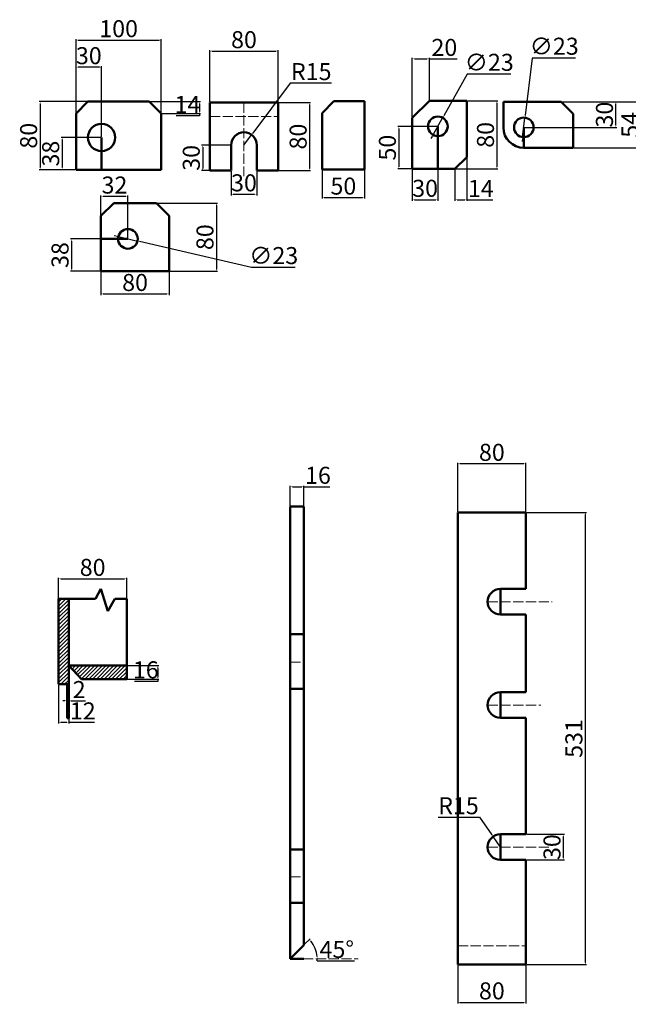
# Model space of a CAD drawing. Units: millimetres. Extents: x 1372 to 2780, y 1459 to 2779.
# Tile 1 of 2: x 1372 to 2087, y 1520 to 2676. Entities that reach past the tile are written whole.
import ezdxf

# ---------------------------------------------------------------- set-up
doc = ezdxf.new("R2010")
doc.units = ezdxf.units.MM
doc.linetypes.add('ACAD_ISO02W100', pattern=[15, 12, -3])
for name, color, linetype, lineweight in [('M-CNTR', 1, 'ACAD_ISO02W100', 18), ('M-DIMS', 2, 'Continuous', 25), ('M-HATC', 8, 'Continuous', 18), ('M-OUTL', 7, 'Continuous', 50)]:
    doc.layers.add(name, color=color, linetype=linetype, lineweight=lineweight)
doc.styles.get("Standard").update_dxf_attribs({"font": 'arial.ttf'})
doc.dimstyles.new('ISO-25', dxfattribs={"dimtxt": 20, "dimasz": 2.5, "dimexe": 1.25, "dimexo": 0.625, "dimtad": 1, "dimtoh": 1, "dimdec": 0, "dimtxsty": 'Standard', "dimcen": 2.5, "dimadec": 0, "dimazin": 0, "dimtfac": 1, "dimtdec": 0, "dimtmove": 0, "dimatfit": 3, "dimfxl": 1, "dimarcsym": 0})

# ---------------------------------------------------------------- blocks, each defined once
blk = doc.blocks.new('*D1')
at = {"layer": 'Defpoints', "color": 0, "transparency": 16777216}
for p in [(1705.8, 2128.1), (1689.8, 2105), (1705.8, 2105)]:
    blk.add_point(p, dxfattribs=at)
at = {"layer": 'M-DIMS', "color": 0, "lineweight": -2, "transparency": 16777216}
for p, q in [((1689.8, 2105.7), (1689.8, 2129.3)), ((1692.3, 2128.1), (1703.3, 2128.1)), ((1705.8, 2105.7), (1705.8, 2129.3)), ((1705.8, 2128.1), (1736.3, 2128.1))]:
    blk.add_line(p, q, dxfattribs=at)
at = {"layer": 'M-DIMS', "color": 0, "transparency": 16777216}
for points in [[(1692.3, 2128.5), (1692.3, 2127.7), (1689.8, 2128.1)], [(1703.3, 2128.5), (1703.3, 2127.7), (1705.8, 2128.1)]]:
    blk.add_solid(points, dxfattribs=at)
at = {"layer": 'M-DIMS', "color": 0, "transparency": 16777216, "insert": (1722.3, 2138.9), "char_height": 20, "attachment_point": 5}
blk.add_mtext('16', dxfattribs=at)
blk = doc.blocks.new('*D2')
at = {"layer": 'Defpoints', "color": 0, "transparency": 16777216}
for p in [(1705.8, 1590), (1717.1, 1589.8), (1689.8, 1574), (1689.8, 1574), (1769.4, 1574)]:
    blk.add_point(p, dxfattribs=at)
at = {"layer": 'M-DIMS', "color": 0, "lineweight": -2, "transparency": 16777216}
for p, q in [((1706.2, 1590.5), (1713, 1597.2)), ((1721.3, 1571.6), (1765.1, 1571.6))]:
    blk.add_line(p, q, dxfattribs=at)
for start, end in [(4.5402, 40.4598), (355.4598, 360)]:
    blk.add_arc((1689.8, 1574), 31.6, start, end, dxfattribs=at)
at = {"layer": 'M-DIMS', "color": 0, "transparency": 16777216}
for points in [[(1713.5, 1594.2), (1714.1, 1594.8), (1712.1, 1596.4)], [(1721.7, 1576.6), (1720.8, 1576.5), (1721.4, 1574)]]:
    blk.add_solid(points, dxfattribs=at)
at = {"layer": 'M-DIMS', "color": 0, "transparency": 16777216, "insert": (1744.4, 1582.3), "char_height": 20, "attachment_point": 5}
blk.add_mtext('45°', dxfattribs=at)
blk = doc.blocks.new('*D3')
at = {"layer": 'Defpoints', "color": 0, "transparency": 16777216}
for p in [(1497.7, 2019.9), (1417.7, 1996.3), (1497.7, 1996.3)]:
    blk.add_point(p, dxfattribs=at)
at = {"layer": 'M-DIMS', "color": 0, "lineweight": -2, "transparency": 16777216}
for p, q in [((1417.7, 1996.9), (1417.7, 2021.2)), ((1420.2, 2019.9), (1495.2, 2019.9)), ((1497.7, 1996.9), (1497.7, 2021.2))]:
    blk.add_line(p, q, dxfattribs=at)
at = {"layer": 'M-DIMS', "color": 0, "transparency": 16777216}
for points in [[(1420.2, 2020.3), (1420.2, 2019.5), (1417.7, 2019.9)], [(1495.2, 2020.3), (1495.2, 2019.5), (1497.7, 2019.9)]]:
    blk.add_solid(points, dxfattribs=at)
at = {"layer": 'M-DIMS', "color": 0, "transparency": 16777216, "insert": (1457.7, 2030.8), "char_height": 20, "attachment_point": 5}
blk.add_mtext('80', dxfattribs=at)
blk = doc.blocks.new('*D4')
at = {"layer": 'Defpoints', "color": 0, "transparency": 16777216}
for p in [(1497.7, 1918.1), (1497.7, 1902.1), (1534.1, 1902.1)]:
    blk.add_point(p, dxfattribs=at)
at = {"layer": 'M-DIMS', "color": 0, "lineweight": -2, "transparency": 16777216}
for p, q in [((1498.3, 1918.1), (1535.3, 1918.1)), ((1534.1, 1915.6), (1534.1, 1904.6)), ((1498.3, 1902.1), (1535.3, 1902.1)), ((1534.1, 1899.6), (1506.7, 1899.6)), ((1534.1, 1902.1), (1534.1, 1899.6))]:
    blk.add_line(p, q, dxfattribs=at)
at = {"layer": 'M-DIMS', "color": 0, "transparency": 16777216}
for points in [[(1533.7, 1915.6), (1534.5, 1915.6), (1534.1, 1918.1)], [(1533.7, 1904.6), (1534.5, 1904.6), (1534.1, 1902.1)]]:
    blk.add_solid(points, dxfattribs=at)
at = {"layer": 'M-DIMS', "color": 0, "transparency": 16777216, "insert": (1520.1, 1910.5), "char_height": 20, "attachment_point": 5}
blk.add_mtext('16', dxfattribs=at)
blk = doc.blocks.new('*D5')
at = {"layer": 'Defpoints', "color": 0, "transparency": 16777216}
for p in [(1417.7, 1896.3), (1429.7, 1896.3), (1429.7, 1851.6)]:
    blk.add_point(p, dxfattribs=at)
at = {"layer": 'M-DIMS', "color": 0, "lineweight": -2, "transparency": 16777216}
for p, q in [((1417.7, 1895.7), (1417.7, 1850.3)), ((1429.7, 1895.7), (1429.7, 1850.3)), ((1420.2, 1851.6), (1427.2, 1851.6)), ((1429.7, 1851.6), (1460, 1851.6))]:
    blk.add_line(p, q, dxfattribs=at)
at = {"layer": 'M-DIMS', "color": 0, "transparency": 16777216}
for points in [[(1420.2, 1852), (1420.2, 1851.2), (1417.7, 1851.6)], [(1427.2, 1852), (1427.2, 1851.2), (1429.7, 1851.6)]]:
    blk.add_solid(points, dxfattribs=at)
at = {"layer": 'M-DIMS', "color": 0, "transparency": 16777216, "insert": (1446.1, 1862.3), "char_height": 20, "attachment_point": 5}
blk.add_mtext('12', dxfattribs=at)
blk = doc.blocks.new('*D6')
at = {"layer": 'Defpoints', "color": 0, "transparency": 16777216}
for p in [(1429.7, 1876.8), (1427.7, 1856.3), (1429.7, 1856.3)]:
    blk.add_point(p, dxfattribs=at)
at = {"layer": 'M-DIMS', "color": 0, "lineweight": -2, "transparency": 16777216}
for p, q in [((1425.2, 1876.8), (1422.7, 1876.8)), ((1427.7, 1856.9), (1427.7, 1878)), ((1427.7, 1876.8), (1429.7, 1876.8)), ((1429.7, 1856.9), (1429.7, 1878)), ((1432.2, 1876.8), (1449.2, 1876.8))]:
    blk.add_line(p, q, dxfattribs=at)
at = {"layer": 'M-DIMS', "color": 0, "transparency": 16777216}
for points in [[(1425.2, 1877.2), (1425.2, 1876.3), (1427.7, 1876.8)], [(1432.2, 1877.2), (1432.2, 1876.3), (1429.7, 1876.8)]]:
    blk.add_solid(points, dxfattribs=at)
at = {"layer": 'M-DIMS', "color": 0, "transparency": 16777216, "insert": (1441.9, 1887.4), "char_height": 20, "attachment_point": 5}
blk.add_mtext('2', dxfattribs=at)
blk = doc.blocks.new('*D7')
at = {"layer": 'Defpoints', "color": 0, "transparency": 16777216}
for p in [(1886.5, 1567), (1966.5, 1567), (1966.5, 1522.7)]:
    blk.add_point(p, dxfattribs=at)
at = {"layer": 'M-DIMS', "color": 0, "lineweight": -2, "transparency": 16777216}
for p, q in [((1886.5, 1566.4), (1886.5, 1521.5)), ((1966.5, 1566.4), (1966.5, 1521.5)), ((1889, 1522.7), (1964, 1522.7))]:
    blk.add_line(p, q, dxfattribs=at)
at = {"layer": 'M-DIMS', "color": 0, "transparency": 16777216}
for points in [[(1889, 1523.1), (1889, 1522.3), (1886.5, 1522.7)], [(1964, 1523.1), (1964, 1522.3), (1966.5, 1522.7)]]:
    blk.add_solid(points, dxfattribs=at)
at = {"layer": 'M-DIMS', "color": 0, "transparency": 16777216, "insert": (1926.5, 1533.6), "char_height": 20, "attachment_point": 5}
blk.add_mtext('80', dxfattribs=at)
blk = doc.blocks.new('*D8')
at = {"layer": 'Defpoints', "color": 0, "transparency": 16777216}
for p in [(1966.5, 2098), (1966.5, 1567), (2036.2, 1567)]:
    blk.add_point(p, dxfattribs=at)
at = {"layer": 'M-DIMS', "color": 0, "lineweight": -2, "transparency": 16777216}
for p, q in [((1967.1, 2098), (2037.5, 2098)), ((2036.2, 2095.5), (2036.2, 1569.5)), ((1967.1, 1567), (2037.5, 1567))]:
    blk.add_line(p, q, dxfattribs=at)
at = {"layer": 'M-DIMS', "color": 0, "transparency": 16777216}
for points in [[(2035.8, 2095.5), (2036.7, 2095.5), (2036.2, 2098)], [(2035.8, 1569.5), (2036.7, 1569.5), (2036.2, 1567)]]:
    blk.add_solid(points, dxfattribs=at)
at = {"layer": 'M-DIMS', "color": 0, "transparency": 16777216, "insert": (2025.4, 1832.5), "char_height": 20, "attachment_point": 5, "rotation": 90}
blk.add_mtext('531', dxfattribs=at)
blk = doc.blocks.new('*D9')
at = {"layer": 'Defpoints', "color": 0, "transparency": 16777216}
for p in [(1966.5, 1720), (2010.6, 1720), (1966.5, 1690)]:
    blk.add_point(p, dxfattribs=at)
at = {"layer": 'M-DIMS', "color": 0, "lineweight": -2, "transparency": 16777216}
for p, q in [((1967.1, 1720), (2011.8, 1720)), ((2010.6, 1692.5), (2010.6, 1717.5)), ((1967.1, 1690), (2011.8, 1690))]:
    blk.add_line(p, q, dxfattribs=at)
at = {"layer": 'M-DIMS', "color": 0, "transparency": 16777216}
for points in [[(2010.1, 1717.5), (2011, 1717.5), (2010.6, 1720)], [(2010.1, 1692.5), (2011, 1692.5), (2010.6, 1690)]]:
    blk.add_solid(points, dxfattribs=at)
at = {"layer": 'M-DIMS', "color": 0, "transparency": 16777216, "insert": (1999.7, 1705), "char_height": 20, "attachment_point": 5, "rotation": 90}
blk.add_mtext('30', dxfattribs=at)
blk = doc.blocks.new('*D10')
at = {"layer": 'Defpoints', "color": 0, "transparency": 16777216}
for p in [(1927.9, 1717.3), (1936.5, 1705)]:
    blk.add_point(p, dxfattribs=at)
at = {"layer": 'M-DIMS', "color": 0, "lineweight": -2, "transparency": 16777216}
for p, q in [((1863.3, 1740.1), (1911.9, 1740.1)), ((1911.9, 1740.1), (1926.5, 1719.3)), ((1936.5, 1705), (1927.9, 1717.3))]:
    blk.add_line(p, q, dxfattribs=at)
at = {"layer": 'M-DIMS', "color": 0, "transparency": 16777216}
blk.add_solid([(1926.8, 1719.6), (1926.1, 1719.1), (1927.9, 1717.3)], dxfattribs=at)
at = {"layer": 'M-DIMS', "color": 0, "transparency": 16777216, "insert": (1887.3, 1751), "char_height": 20, "attachment_point": 5}
blk.add_mtext('R15', dxfattribs=at)
blk = doc.blocks.new('*D11')
at = {"layer": 'Defpoints', "color": 0, "transparency": 16777216}
for p in [(1886.5, 2155), (1886.5, 2098), (1966.5, 2098)]:
    blk.add_point(p, dxfattribs=at)
at = {"layer": 'M-DIMS', "color": 0, "lineweight": -2, "transparency": 16777216}
for p, q in [((1886.5, 2098.6), (1886.5, 2156.3)), ((1964, 2155), (1889, 2155)), ((1966.5, 2098.6), (1966.5, 2156.3))]:
    blk.add_line(p, q, dxfattribs=at)
at = {"layer": 'M-DIMS', "color": 0, "transparency": 16777216}
for points in [[(1889, 2155.4), (1889, 2154.6), (1886.5, 2155)], [(1964, 2155.4), (1964, 2154.6), (1966.5, 2155)]]:
    blk.add_solid(points, dxfattribs=at)
at = {"layer": 'M-DIMS', "color": 0, "transparency": 16777216, "insert": (1926.5, 2165.9), "char_height": 20, "attachment_point": 5}
blk.add_mtext('80', dxfattribs=at)
blk = doc.blocks.new('*D27')
at = {"layer": 'Defpoints', "color": 0, "transparency": 16777216}
for p in [(1467.5, 2381.1), (1547.5, 2381.1), (1547.5, 2354.5)]:
    blk.add_point(p, dxfattribs=at)
at = {"layer": 'M-DIMS', "color": 0, "lineweight": -2, "transparency": 16777216}
for p, q in [((1467.5, 2380.5), (1467.5, 2353.2)), ((1547.5, 2380.5), (1547.5, 2353.2)), ((1470, 2354.5), (1545, 2354.5))]:
    blk.add_line(p, q, dxfattribs=at)
at = {"layer": 'M-DIMS', "color": 0, "transparency": 16777216}
for points in [[(1470, 2354.9), (1470, 2354.1), (1467.5, 2354.5)], [(1545, 2354.9), (1545, 2354.1), (1547.5, 2354.5)]]:
    blk.add_solid(points, dxfattribs=at)
at = {"layer": 'M-DIMS', "color": 0, "transparency": 16777216, "insert": (1507.5, 2365.3), "char_height": 20, "attachment_point": 5}
blk.add_mtext('80', dxfattribs=at)
blk = doc.blocks.new('*D28')
at = {"layer": 'Defpoints', "color": 0, "transparency": 16777216}
for p in [(1499.1, 2419.1), (1432.9, 2381.1), (1467.5, 2381.1)]:
    blk.add_point(p, dxfattribs=at)
at = {"layer": 'M-DIMS', "color": 0, "lineweight": -2, "transparency": 16777216}
for p, q in [((1498.5, 2419.1), (1431.6, 2419.1)), ((1432.9, 2416.6), (1432.9, 2383.6)), ((1466.9, 2381.1), (1431.6, 2381.1))]:
    blk.add_line(p, q, dxfattribs=at)
at = {"layer": 'M-DIMS', "color": 0, "transparency": 16777216}
for points in [[(1432.4, 2416.6), (1433.3, 2416.6), (1432.9, 2419.1)], [(1432.4, 2383.6), (1433.3, 2383.6), (1432.9, 2381.1)]]:
    blk.add_solid(points, dxfattribs=at)
at = {"layer": 'M-DIMS', "color": 0, "transparency": 16777216, "insert": (1422, 2400.1), "char_height": 20, "attachment_point": 5, "rotation": 90}
blk.add_mtext('38', dxfattribs=at)
blk = doc.blocks.new('*D29')
at = {"layer": 'Defpoints', "color": 0, "transparency": 16777216}
for p in [(1467.5, 2468.9), (1467.5, 2446.1), (1499.1, 2419.1)]:
    blk.add_point(p, dxfattribs=at)
at = {"layer": 'M-DIMS', "color": 0, "lineweight": -2, "transparency": 16777216}
for p, q in [((1467.5, 2446.7), (1467.5, 2470.1)), ((1496.6, 2468.9), (1470, 2468.9)), ((1499.1, 2419.7), (1499.1, 2470.1))]:
    blk.add_line(p, q, dxfattribs=at)
at = {"layer": 'M-DIMS', "color": 0, "transparency": 16777216}
for points in [[(1470, 2469.3), (1470, 2468.5), (1467.5, 2468.9)], [(1496.6, 2469.3), (1496.6, 2468.5), (1499.1, 2468.9)]]:
    blk.add_solid(points, dxfattribs=at)
at = {"layer": 'M-DIMS', "color": 0, "transparency": 16777216, "insert": (1483.3, 2479.7), "char_height": 20, "attachment_point": 5}
blk.add_mtext('32', dxfattribs=at)
blk = doc.blocks.new('*D30')
at = {"layer": 'Defpoints', "color": 0, "transparency": 16777216}
for p in [(1532.5, 2461.1), (1547.5, 2381.1), (1603, 2381.1)]:
    blk.add_point(p, dxfattribs=at)
at = {"layer": 'M-DIMS', "color": 0, "lineweight": -2, "transparency": 16777216}
for p, q in [((1533.1, 2461.1), (1604.3, 2461.1)), ((1603, 2458.6), (1603, 2383.6)), ((1548.1, 2381.1), (1604.3, 2381.1))]:
    blk.add_line(p, q, dxfattribs=at)
at = {"layer": 'M-DIMS', "color": 0, "transparency": 16777216}
for points in [[(1602.6, 2458.6), (1603.4, 2458.6), (1603, 2461.1)], [(1602.6, 2383.6), (1603.4, 2383.6), (1603, 2381.1)]]:
    blk.add_solid(points, dxfattribs=at)
at = {"layer": 'M-DIMS', "color": 0, "transparency": 16777216, "insert": (1592.2, 2421.1), "char_height": 20, "attachment_point": 5, "rotation": 90}
blk.add_mtext('80', dxfattribs=at)
blk = doc.blocks.new('*D31')
at = {"layer": 'Defpoints', "color": 0, "transparency": 16777216}
for p in [(1487.9, 2421.7), (1510.3, 2416.5)]:
    blk.add_point(p, dxfattribs=at)
at = {"layer": 'M-DIMS', "color": 0, "lineweight": -2, "transparency": 16777216}
for p, q in [((1485.5, 2422.2), (1483.1, 2422.8)), ((1487.9, 2421.7), (1510.3, 2416.5)), ((1644.4, 2385.5), (1512.8, 2415.9)), ((1695.5, 2385.5), (1644.4, 2385.5))]:
    blk.add_line(p, q, dxfattribs=at)
at = {"layer": 'M-DIMS', "color": 0, "transparency": 16777216}
for points in [[(1485.6, 2422.6), (1485.4, 2421.8), (1487.9, 2421.7)], [(1512.9, 2416.3), (1512.7, 2415.5), (1510.3, 2416.5)]]:
    blk.add_solid(points, dxfattribs=at)
at = {"layer": 'M-DIMS', "color": 0, "transparency": 16777216, "insert": (1670.3, 2396.9), "char_height": 20, "attachment_point": 5}
blk.add_mtext('∅23', dxfattribs=at)
blk = doc.blocks.new('*D32')
at = {"layer": 'Defpoints', "color": 0, "transparency": 16777216}
for p in [(1438.2, 2620.8), (1438.2, 2533.2), (1468.2, 2538.2)]:
    blk.add_point(p, dxfattribs=at)
at = {"layer": 'M-DIMS', "color": 0, "lineweight": -2, "transparency": 16777216}
for p, q in [((1438.2, 2533.8), (1438.2, 2622)), ((1465.7, 2620.8), (1440.7, 2620.8)), ((1468.2, 2538.8), (1468.2, 2622))]:
    blk.add_line(p, q, dxfattribs=at)
at = {"layer": 'M-DIMS', "color": 0, "transparency": 16777216}
for points in [[(1440.7, 2621.2), (1440.7, 2620.4), (1438.2, 2620.8)], [(1465.7, 2621.2), (1465.7, 2620.4), (1468.2, 2620.8)]]:
    blk.add_solid(points, dxfattribs=at)
at = {"layer": 'M-DIMS', "color": 0, "transparency": 16777216, "insert": (1453.2, 2631.6), "char_height": 20, "attachment_point": 5}
blk.add_mtext('30', dxfattribs=at)
blk = doc.blocks.new('*D33')
at = {"layer": 'Defpoints', "color": 0, "transparency": 16777216}
for p in [(1524.2, 2580.2), (1538.2, 2566.2), (1583, 2566.2)]:
    blk.add_point(p, dxfattribs=at)
at = {"layer": 'M-DIMS', "color": 0, "lineweight": -2, "transparency": 16777216}
for p, q in [((1524.8, 2580.2), (1584.2, 2580.2)), ((1583, 2577.7), (1583, 2568.7)), ((1538.8, 2566.2), (1584.2, 2566.2)), ((1583, 2563.7), (1555.6, 2563.7)), ((1583, 2566.2), (1583, 2563.7))]:
    blk.add_line(p, q, dxfattribs=at)
at = {"layer": 'M-DIMS', "color": 0, "transparency": 16777216}
for points in [[(1582.5, 2577.7), (1583.4, 2577.7), (1583, 2580.2)], [(1582.5, 2568.7), (1583.4, 2568.7), (1583, 2566.2)]]:
    blk.add_solid(points, dxfattribs=at)
at = {"layer": 'M-DIMS', "color": 0, "transparency": 16777216, "insert": (1569, 2574.3), "char_height": 20, "attachment_point": 5}
blk.add_mtext('14', dxfattribs=at)
blk = doc.blocks.new('*D34')
at = {"layer": 'Defpoints', "color": 0, "transparency": 16777216}
for p in [(1452.2, 2580.2), (1396, 2500.2), (1438.2, 2500.2)]:
    blk.add_point(p, dxfattribs=at)
at = {"layer": 'M-DIMS', "color": 0, "lineweight": -2, "transparency": 16777216}
for p, q in [((1451.6, 2580.2), (1394.7, 2580.2)), ((1396, 2577.7), (1396, 2502.7)), ((1437.6, 2500.2), (1394.7, 2500.2))]:
    blk.add_line(p, q, dxfattribs=at)
at = {"layer": 'M-DIMS', "color": 0, "transparency": 16777216}
for points in [[(1395.6, 2577.7), (1396.4, 2577.7), (1396, 2580.2)], [(1395.6, 2502.7), (1396.4, 2502.7), (1396, 2500.2)]]:
    blk.add_solid(points, dxfattribs=at)
at = {"layer": 'M-DIMS', "color": 0, "transparency": 16777216, "insert": (1385.1, 2540.2), "char_height": 20, "attachment_point": 5, "rotation": 90}
blk.add_mtext('80', dxfattribs=at)
blk = doc.blocks.new('*D35')
at = {"layer": 'Defpoints', "color": 0, "transparency": 16777216}
for p in [(1468.2, 2538.2), (1421.9, 2500.2), (1438.2, 2500.2)]:
    blk.add_point(p, dxfattribs=at)
at = {"layer": 'M-DIMS', "color": 0, "lineweight": -2, "transparency": 16777216}
for p, q in [((1467.6, 2538.2), (1420.6, 2538.2)), ((1421.9, 2535.7), (1421.9, 2502.7)), ((1437.6, 2500.2), (1420.6, 2500.2))]:
    blk.add_line(p, q, dxfattribs=at)
at = {"layer": 'M-DIMS', "color": 0, "transparency": 16777216}
for points in [[(1421.4, 2535.7), (1422.3, 2535.7), (1421.9, 2538.2)], [(1421.4, 2502.7), (1422.3, 2502.7), (1421.9, 2500.2)]]:
    blk.add_solid(points, dxfattribs=at)
at = {"layer": 'M-DIMS', "color": 0, "transparency": 16777216, "insert": (1411, 2519.2), "char_height": 20, "attachment_point": 5, "rotation": 90}
blk.add_mtext('38', dxfattribs=at)
blk = doc.blocks.new('*D36')
at = {"layer": 'Defpoints', "color": 0, "transparency": 16777216}
for p in [(1538.2, 2652.5), (1438.2, 2500.2), (1538.2, 2500.2)]:
    blk.add_point(p, dxfattribs=at)
at = {"layer": 'M-DIMS', "color": 0, "lineweight": -2, "transparency": 16777216}
for p, q in [((1438.2, 2500.8), (1438.2, 2653.7)), ((1440.7, 2652.5), (1535.7, 2652.5)), ((1538.2, 2500.8), (1538.2, 2653.7))]:
    blk.add_line(p, q, dxfattribs=at)
at = {"layer": 'M-DIMS', "color": 0, "transparency": 16777216}
for points in [[(1440.7, 2652.9), (1440.7, 2652.1), (1438.2, 2652.5)], [(1535.7, 2652.9), (1535.7, 2652.1), (1538.2, 2652.5)]]:
    blk.add_solid(points, dxfattribs=at)
at = {"layer": 'M-DIMS', "color": 0, "transparency": 16777216, "insert": (1488.2, 2663.3), "char_height": 20, "attachment_point": 5}
blk.add_mtext('100', dxfattribs=at)
blk = doc.blocks.new('*D37')
at = {"layer": 'Defpoints', "color": 0, "transparency": 16777216}
for p in [(1675.4, 2639.6), (1595.4, 2579.2), (1675.4, 2579.2)]:
    blk.add_point(p, dxfattribs=at)
at = {"layer": 'M-DIMS', "color": 0, "lineweight": -2, "transparency": 16777216}
for p, q in [((1595.4, 2579.8), (1595.4, 2640.8)), ((1597.9, 2639.6), (1672.9, 2639.6)), ((1675.4, 2579.8), (1675.4, 2640.8))]:
    blk.add_line(p, q, dxfattribs=at)
at = {"layer": 'M-DIMS', "color": 0, "transparency": 16777216}
for points in [[(1597.9, 2640), (1597.9, 2639.1), (1595.4, 2639.6)], [(1672.9, 2640), (1672.9, 2639.1), (1675.4, 2639.6)]]:
    blk.add_solid(points, dxfattribs=at)
at = {"layer": 'M-DIMS', "color": 0, "transparency": 16777216, "insert": (1635.4, 2650.4), "char_height": 20, "attachment_point": 5}
blk.add_mtext('80', dxfattribs=at)
blk = doc.blocks.new('*D38')
at = {"layer": 'Defpoints', "color": 0, "transparency": 16777216}
for p in [(1675.4, 2579.2), (1675.4, 2499.2), (1712.4, 2499.2)]:
    blk.add_point(p, dxfattribs=at)
at = {"layer": 'M-DIMS', "color": 0, "lineweight": -2, "transparency": 16777216}
for p, q in [((1676, 2579.2), (1713.7, 2579.2)), ((1712.4, 2576.7), (1712.4, 2501.7)), ((1676, 2499.2), (1713.7, 2499.2))]:
    blk.add_line(p, q, dxfattribs=at)
at = {"layer": 'M-DIMS', "color": 0, "transparency": 16777216}
for points in [[(1712, 2576.7), (1712.8, 2576.7), (1712.4, 2579.2)], [(1712, 2501.7), (1712.8, 2501.7), (1712.4, 2499.2)]]:
    blk.add_solid(points, dxfattribs=at)
at = {"layer": 'M-DIMS', "color": 0, "transparency": 16777216, "insert": (1701.6, 2539.2), "char_height": 20, "attachment_point": 5, "rotation": 90}
blk.add_mtext('80', dxfattribs=at)
blk = doc.blocks.new('*D39')
at = {"layer": 'Defpoints', "color": 0, "transparency": 16777216}
for p in [(1620.4, 2499.2), (1650.4, 2499.2), (1650.4, 2471.5)]:
    blk.add_point(p, dxfattribs=at)
at = {"layer": 'M-DIMS', "color": 0, "lineweight": -2, "transparency": 16777216}
for p, q in [((1620.4, 2498.6), (1620.4, 2470.2)), ((1650.4, 2498.6), (1650.4, 2470.2)), ((1622.9, 2471.5), (1647.9, 2471.5))]:
    blk.add_line(p, q, dxfattribs=at)
at = {"layer": 'M-DIMS', "color": 0, "transparency": 16777216}
for points in [[(1622.9, 2471.9), (1622.9, 2471.1), (1620.4, 2471.5)], [(1647.9, 2471.9), (1647.9, 2471.1), (1650.4, 2471.5)]]:
    blk.add_solid(points, dxfattribs=at)
at = {"layer": 'M-DIMS', "color": 0, "transparency": 16777216, "insert": (1635.4, 2482.3), "char_height": 20, "attachment_point": 5}
blk.add_mtext('30', dxfattribs=at)
blk = doc.blocks.new('*D40')
at = {"layer": 'Defpoints', "color": 0, "transparency": 16777216}
for p in [(1644.3, 2541.2), (1635.4, 2529.2)]:
    blk.add_point(p, dxfattribs=at)
at = {"layer": 'M-DIMS', "color": 0, "lineweight": -2, "transparency": 16777216}
for p, q in [((1689.8, 2602.1), (1645.8, 2543.2)), ((1738.3, 2602.1), (1689.8, 2602.1)), ((1635.4, 2529.2), (1644.3, 2541.2))]:
    blk.add_line(p, q, dxfattribs=at)
at = {"layer": 'M-DIMS', "color": 0, "transparency": 16777216}
blk.add_solid([(1645.5, 2543.5), (1646.2, 2543), (1644.3, 2541.2)], dxfattribs=at)
at = {"layer": 'M-DIMS', "color": 0, "transparency": 16777216, "insert": (1714.4, 2612.9), "char_height": 20, "attachment_point": 5}
blk.add_mtext('R15', dxfattribs=at)
blk = doc.blocks.new('*D41')
at = {"layer": 'Defpoints', "color": 0, "transparency": 16777216}
for p in [(1620.4, 2529.2), (1586.9, 2499.2), (1620.4, 2499.2)]:
    blk.add_point(p, dxfattribs=at)
at = {"layer": 'M-DIMS', "color": 0, "lineweight": -2, "transparency": 16777216}
for p, q in [((1619.7, 2529.2), (1585.7, 2529.2)), ((1586.9, 2526.7), (1586.9, 2501.7)), ((1619.7, 2499.2), (1585.7, 2499.2))]:
    blk.add_line(p, q, dxfattribs=at)
at = {"layer": 'M-DIMS', "color": 0, "transparency": 16777216}
for points in [[(1586.5, 2526.7), (1587.3, 2526.7), (1586.9, 2529.2)], [(1586.5, 2501.7), (1587.3, 2501.7), (1586.9, 2499.2)]]:
    blk.add_solid(points, dxfattribs=at)
at = {"layer": 'M-DIMS', "color": 0, "transparency": 16777216, "insert": (1576.1, 2514.2), "char_height": 20, "attachment_point": 5, "rotation": 90}
blk.add_mtext('30', dxfattribs=at)
blk = doc.blocks.new('*D42')
at = {"layer": 'Defpoints', "color": 0, "transparency": 16777216}
for p in [(1727.1, 2500.6), (1777.1, 2500.6), (1777.1, 2467.6)]:
    blk.add_point(p, dxfattribs=at)
at = {"layer": 'M-DIMS', "color": 0, "lineweight": -2, "transparency": 16777216}
for p, q in [((1727.1, 2500), (1727.1, 2466.4)), ((1777.1, 2500), (1777.1, 2466.4)), ((1729.6, 2467.6), (1774.6, 2467.6))]:
    blk.add_line(p, q, dxfattribs=at)
at = {"layer": 'M-DIMS', "color": 0, "transparency": 16777216}
for points in [[(1729.6, 2468), (1729.6, 2467.2), (1727.1, 2467.6)], [(1774.6, 2468), (1774.6, 2467.2), (1777.1, 2467.6)]]:
    blk.add_solid(points, dxfattribs=at)
at = {"layer": 'M-DIMS', "color": 0, "transparency": 16777216, "insert": (1752.1, 2478.5), "char_height": 20, "attachment_point": 5}
blk.add_mtext('50', dxfattribs=at)
blk = doc.blocks.new('*D43')
at = {"layer": 'Defpoints', "color": 0, "transparency": 16777216}
for p in [(1833.1, 2501.2), (1863.1, 2501.2), (1863.1, 2465)]:
    blk.add_point(p, dxfattribs=at)
at = {"layer": 'M-DIMS', "color": 0, "lineweight": -2, "transparency": 16777216}
for p, q in [((1833.1, 2500.6), (1833.1, 2463.8)), ((1863.1, 2500.6), (1863.1, 2463.8)), ((1835.6, 2465), (1860.6, 2465))]:
    blk.add_line(p, q, dxfattribs=at)
at = {"layer": 'M-DIMS', "color": 0, "transparency": 16777216}
for points in [[(1835.6, 2465.4), (1835.6, 2464.6), (1833.1, 2465)], [(1860.6, 2465.4), (1860.6, 2464.6), (1863.1, 2465)]]:
    blk.add_solid(points, dxfattribs=at)
at = {"layer": 'M-DIMS', "color": 0, "transparency": 16777216, "insert": (1848.1, 2475.9), "char_height": 20, "attachment_point": 5}
blk.add_mtext('30', dxfattribs=at)
blk = doc.blocks.new('*D44')
at = {"layer": 'Defpoints', "color": 0, "transparency": 16777216}
for p in [(1853.1, 2630.5), (1853.1, 2581.2), (1833.1, 2561.2)]:
    blk.add_point(p, dxfattribs=at)
at = {"layer": 'M-DIMS', "color": 0, "lineweight": -2, "transparency": 16777216}
for p, q in [((1833.1, 2561.9), (1833.1, 2631.8)), ((1835.6, 2630.5), (1850.6, 2630.5)), ((1853.1, 2581.9), (1853.1, 2631.8)), ((1853.1, 2630.5), (1885.8, 2630.5))]:
    blk.add_line(p, q, dxfattribs=at)
at = {"layer": 'M-DIMS', "color": 0, "transparency": 16777216}
for points in [[(1835.6, 2630.9), (1835.6, 2630.1), (1833.1, 2630.5)], [(1850.6, 2630.9), (1850.6, 2630.1), (1853.1, 2630.5)]]:
    blk.add_solid(points, dxfattribs=at)
at = {"layer": 'M-DIMS', "color": 0, "transparency": 16777216, "insert": (1870.7, 2641.3), "char_height": 20, "attachment_point": 5}
blk.add_mtext('20', dxfattribs=at)
blk = doc.blocks.new('*D45')
at = {"layer": 'Defpoints', "color": 0, "transparency": 16777216}
for p in [(1897.1, 2515.2), (1883.1, 2501.2), (1897.1, 2465)]:
    blk.add_point(p, dxfattribs=at)
at = {"layer": 'M-DIMS', "color": 0, "lineweight": -2, "transparency": 16777216}
for p, q in [((1897.1, 2514.6), (1897.1, 2463.8)), ((1883.1, 2500.6), (1883.1, 2463.8)), ((1885.6, 2465), (1894.6, 2465)), ((1897.1, 2465), (1927.5, 2465))]:
    blk.add_line(p, q, dxfattribs=at)
at = {"layer": 'M-DIMS', "color": 0, "transparency": 16777216}
for points in [[(1885.6, 2465.4), (1885.6, 2464.6), (1883.1, 2465)], [(1894.6, 2465.4), (1894.6, 2464.6), (1897.1, 2465)]]:
    blk.add_solid(points, dxfattribs=at)
at = {"layer": 'M-DIMS', "color": 0, "transparency": 16777216, "insert": (1913.6, 2475.7), "char_height": 20, "attachment_point": 5}
blk.add_mtext('14', dxfattribs=at)
blk = doc.blocks.new('*D46')
at = {"layer": 'Defpoints', "color": 0, "transparency": 16777216}
for p in [(1897.1, 2581.2), (1883.1, 2501.2), (1932.4, 2501.2)]:
    blk.add_point(p, dxfattribs=at)
at = {"layer": 'M-DIMS', "color": 0, "lineweight": -2, "transparency": 16777216}
for p, q in [((1897.7, 2581.2), (1933.6, 2581.2)), ((1932.4, 2578.7), (1932.4, 2503.7)), ((1883.7, 2501.2), (1933.6, 2501.2))]:
    blk.add_line(p, q, dxfattribs=at)
at = {"layer": 'M-DIMS', "color": 0, "transparency": 16777216}
for points in [[(1932, 2578.7), (1932.8, 2578.7), (1932.4, 2581.2)], [(1932, 2503.7), (1932.8, 2503.7), (1932.4, 2501.2)]]:
    blk.add_solid(points, dxfattribs=at)
at = {"layer": 'M-DIMS', "color": 0, "transparency": 16777216, "insert": (1921.6, 2541.2), "char_height": 20, "attachment_point": 5, "rotation": 90}
blk.add_mtext('80', dxfattribs=at)
blk = doc.blocks.new('*D47')
at = {"layer": 'Defpoints', "color": 0, "transparency": 16777216}
for p in [(1863.1, 2551.2), (1817.2, 2501.2), (1858.1, 2501.2)]:
    blk.add_point(p, dxfattribs=at)
at = {"layer": 'M-DIMS', "color": 0, "lineweight": -2, "transparency": 16777216}
for p, q in [((1862.5, 2551.2), (1816, 2551.2)), ((1817.2, 2548.7), (1817.2, 2503.7)), ((1857.5, 2501.2), (1816, 2501.2))]:
    blk.add_line(p, q, dxfattribs=at)
at = {"layer": 'M-DIMS', "color": 0, "transparency": 16777216}
for points in [[(1816.8, 2548.7), (1817.6, 2548.7), (1817.2, 2551.2)], [(1816.8, 2503.7), (1817.6, 2503.7), (1817.2, 2501.2)]]:
    blk.add_solid(points, dxfattribs=at)
at = {"layer": 'M-DIMS', "color": 0, "transparency": 16777216, "insert": (1806.4, 2526.2), "char_height": 20, "attachment_point": 5, "rotation": 90}
blk.add_mtext('50', dxfattribs=at)
blk = doc.blocks.new('*D48')
at = {"layer": 'Defpoints', "color": 0, "transparency": 16777216}
for p in [(2008, 2580), (2072.1, 2580), (1964, 2550)]:
    blk.add_point(p, dxfattribs=at)
at = {"layer": 'M-DIMS', "color": 0, "lineweight": -2, "transparency": 16777216}
for p, q in [((2008.6, 2580), (2073.4, 2580)), ((2072.1, 2552.5), (2072.1, 2577.5)), ((1964.6, 2550), (2073.4, 2550))]:
    blk.add_line(p, q, dxfattribs=at)
at = {"layer": 'M-DIMS', "color": 0, "transparency": 16777216}
for points in [[(2071.7, 2577.5), (2072.6, 2577.5), (2072.1, 2580)], [(2071.7, 2552.5), (2072.6, 2552.5), (2072.1, 2550)]]:
    blk.add_solid(points, dxfattribs=at)
at = {"layer": 'M-DIMS', "color": 0, "transparency": 16777216, "insert": (2061.3, 2565), "char_height": 20, "attachment_point": 5, "rotation": 90}
blk.add_mtext('30', dxfattribs=at)
blk = doc.blocks.new('*D49')
at = {"layer": 'Defpoints', "color": 0, "transparency": 16777216}
for p in [(2008, 2580), (2022, 2526), (2102.1, 2526)]:
    blk.add_point(p, dxfattribs=at)
at = {"layer": 'M-DIMS', "color": 0, "lineweight": -2, "transparency": 16777216}
for p, q in [((2008.6, 2580), (2103.3, 2580)), ((2102.1, 2577.5), (2102.1, 2528.5)), ((2022.6, 2526), (2103.3, 2526))]:
    blk.add_line(p, q, dxfattribs=at)
at = {"layer": 'M-DIMS', "color": 0, "transparency": 16777216}
for points in [[(2101.7, 2577.5), (2102.5, 2577.5), (2102.1, 2580)], [(2101.7, 2528.5), (2102.5, 2528.5), (2102.1, 2526)]]:
    blk.add_solid(points, dxfattribs=at)
at = {"layer": 'M-DIMS', "color": 0, "transparency": 16777216, "insert": (2091.3, 2553), "char_height": 20, "attachment_point": 5, "rotation": 90}
blk.add_mtext('54', dxfattribs=at)
blk = doc.blocks.new('*D50')
at = {"layer": 'Defpoints', "color": 0, "transparency": 16777216}
for p in [(1868.7, 2561.3), (1857.4, 2541.2)]:
    blk.add_point(p, dxfattribs=at)
at = {"layer": 'M-DIMS', "color": 0, "lineweight": -2, "transparency": 16777216}
for p, q in [((1897.6, 2612.4), (1870, 2563.4)), ((1948.6, 2612.4), (1897.6, 2612.4)), ((1857.4, 2541.2), (1868.7, 2561.3)), ((1856.2, 2539.1), (1855, 2536.9))]:
    blk.add_line(p, q, dxfattribs=at)
at = {"layer": 'M-DIMS', "color": 0, "transparency": 16777216}
for points in [[(1869.6, 2563.6), (1870.3, 2563.2), (1868.7, 2561.3)], [(1855.8, 2539.3), (1856.6, 2538.9), (1857.4, 2541.2)]]:
    blk.add_solid(points, dxfattribs=at)
at = {"layer": 'M-DIMS', "color": 0, "transparency": 16777216, "insert": (1923.4, 2623.8), "char_height": 20, "attachment_point": 5}
blk.add_mtext('∅23', dxfattribs=at)
blk = doc.blocks.new('*D51')
at = {"layer": 'Defpoints', "color": 0, "transparency": 16777216}
for p in [(1965.3, 2561.4), (1962.6, 2538.6)]:
    blk.add_point(p, dxfattribs=at)
at = {"layer": 'M-DIMS', "color": 0, "lineweight": -2, "transparency": 16777216}
for p, q in [((1973.8, 2631.3), (1965.7, 2563.9)), ((2024.9, 2631.3), (1973.8, 2631.3)), ((1962.6, 2538.6), (1965.3, 2561.4)), ((1962.3, 2536.1), (1962, 2533.6))]:
    blk.add_line(p, q, dxfattribs=at)
at = {"layer": 'M-DIMS', "color": 0, "transparency": 16777216}
for points in [[(1965.2, 2564), (1966.1, 2563.9), (1965.3, 2561.4)], [(1961.9, 2536.2), (1962.7, 2536.1), (1962.6, 2538.6)]]:
    blk.add_solid(points, dxfattribs=at)
at = {"layer": 'M-DIMS', "color": 0, "transparency": 16777216, "insert": (1999.7, 2642.7), "char_height": 20, "attachment_point": 5}
blk.add_mtext('∅23', dxfattribs=at)

msp = doc.modelspace()

# ---------------------------------------------------------------- hatches: boundary and pattern name
at = {"layer": 'M-HATC'}
h = msp.add_hatch(dxfattribs=at)
h.set_pattern_fill('ANSI31', color=256)
h.paths.add_polyline_path([(1429.7, 1996.3), (1417.7, 1996.3), (1417.7, 1896.3), (1429.7, 1896.3), (1429.7, 1918.1), (1429.7, 1918.1), (1429.7, 1918.1)])
h.paths.add_polyline_path([(1497.7, 1918.1), (1429.7, 1918.1), (1429.7, 1918.1), (1444.8, 1902.1), (1497.7, 1902.1)])

# ---------------------------------------------------------------- linework, layer by layer
at = {"layer": 'M-CNTR'}
for p, q in [((1635.4, 2579.2), (1635.4, 2492.6)), ((1595.4, 2562.7), (1675.4, 2562.7)), ((1921.5, 1993.1), (1997.2, 1993.1)), ((1689.8, 1922.3), (1705.8, 1922.3)), ((1921.5, 1871.8), (1983.9, 1871.8)), ((1921.5, 1705), (1996.5, 1705)), ((1689.8, 1670.1), (1705.8, 1670.1)), ((1886.5, 1588.9), (1966.5, 1588.9)), ((1689.8, 1574), (1769.4, 1574))]:
    msp.add_line(p, q, dxfattribs=at)
at = {"layer": 'M-OUTL'}
for p, q in [((1438.2, 2566.2), (1452.2, 2580.2)), ((1452.2, 2580.2), (1524.2, 2580.2)), ((1538.2, 2566.2), (1524.2, 2580.2)), ((1595.4, 2579.2), (1675.4, 2579.2)), ((1595.4, 2499.2), (1595.4, 2579.2)), ((1675.4, 2579.2), (1675.4, 2499.2)), ((1727.1, 2566.6), (1741.1, 2580.6)), ((1777.1, 2580.6), (1741.1, 2580.6)), ((1777.1, 2500.6), (1777.1, 2580.6)), ((1833.1, 2561.2), (1853.1, 2581.2)), ((1897.1, 2581.2), (1853.1, 2581.2)), ((1897.1, 2515.2), (1897.1, 2581.2)), ((1940, 2580), (2008, 2580)), ((1940, 2550), (1940, 2580)), ((2008, 2580), (2022, 2566)), ((1727.1, 2566.6), (1727.1, 2500.6)), ((1438.2, 2500.2), (1438.2, 2566.2)), ((1538.2, 2500.2), (1538.2, 2566.2)), ((1833.1, 2561.2), (1833.1, 2501.2)), ((2022, 2566), (2022, 2526)), ((1863.1, 2501.2), (1863.1, 2551.2)), ((1964, 2526), (1964, 2550)), ((1468.2, 2500.2), (1468.2, 2538.2)), ((1620.4, 2529.2), (1620.4, 2499.2)), ((1650.4, 2499.2), (1650.4, 2529.2)), ((2022, 2526), (1964, 2526)), ((2022, 2526), (1964, 2526)), ((1883.1, 2501.2), (1897.1, 2515.2)), ((1538.2, 2500.2), (1438.2, 2500.2)), ((1438.2, 2500.2), (1468.2, 2500.2)), ((1620.4, 2499.2), (1595.4, 2499.2)), ((1675.4, 2499.2), (1650.4, 2499.2)), ((1727.1, 2500.6), (1777.1, 2500.6)), ((1833.1, 2501.2), (1883.1, 2501.2)), ((1833.1, 2501.2), (1863.1, 2501.2)), ((1467.5, 2446.1), (1482.5, 2461.1)), ((1532.5, 2461.1), (1482.5, 2461.1)), ((1532.5, 2461.1), (1547.5, 2446.1)), ((1467.5, 2446.1), (1467.5, 2381.1)), ((1547.5, 2381.1), (1547.5, 2446.1)), ((1467.5, 2381.1), (1467.5, 2419.1)), ((1467.5, 2419.1), (1499.1, 2419.1)), ((1467.5, 2381.1), (1547.5, 2381.1)), ((1689.8, 2105), (1689.8, 1574)), ((1705.8, 2105), (1689.8, 2105)), ((1705.8, 1590), (1705.8, 2105)), ((1886.5, 2098), (1966.5, 2098)), ((1886.5, 2098), (1886.5, 1567)), ((1966.5, 2008.1), (1966.5, 2098)), ((1461.1, 1996.3), (1467.4, 2008.3)), ((1467.4, 2008.3), (1475.7, 1981.9)), ((1936.5, 2008.1), (1966.5, 2008.1)), ((1936.5, 2008.1), (1936.5, 1978.1)), ((1429.7, 1996.3), (1417.7, 1996.3)), ((1417.7, 1996.3), (1417.7, 1896.3)), ((1429.7, 1896.3), (1429.7, 1996.3)), ((1429.7, 1996.3), (1461.1, 1996.3)), ((1475.7, 1981.9), (1483.7, 1996.3)), ((1497.7, 1996.3), (1483.7, 1996.3)), ((1497.7, 1996.3), (1497.7, 1918.1)), ((1936.5, 1978.1), (1966.5, 1978.1)), ((1966.5, 1886.8), (1966.5, 1978.1)), ((1689.8, 1955.1), (1705.8, 1955.1)), ((1429.7, 1918.1), (1497.7, 1918.1)), ((1444.8, 1902.1), (1429.7, 1918.1)), ((1497.7, 1918.1), (1497.7, 1902.1)), ((1417.7, 1896.3), (1429.7, 1896.3)), ((1427.7, 1856.3), (1427.7, 1896.3)), ((1429.7, 1896.3), (1429.7, 1888.3)), ((1497.7, 1902.1), (1444.8, 1902.1)), ((1429.7, 1888.3), (1429.7, 1856.3)), ((1705.8, 1890.7), (1689.8, 1890.7)), ((1936.5, 1886.8), (1966.5, 1886.8)), ((1936.5, 1886.8), (1936.5, 1856.8)), ((1429.7, 1856.3), (1427.7, 1856.3)), ((1936.5, 1856.8), (1966.5, 1856.8)), ((1966.5, 1720), (1966.5, 1856.8)), ((1936.5, 1720), (1966.5, 1720)), ((1936.5, 1720), (1936.5, 1690)), ((1689.8, 1702), (1705.8, 1702)), ((1936.5, 1690), (1966.5, 1690)), ((1966.5, 1567), (1966.5, 1690)), ((1705.8, 1639.5), (1689.8, 1639.5)), ((1689.8, 1574), (1705.8, 1590)), ((1689.8, 1574), (1705.8, 1574)), ((1886.5, 1567), (1966.5, 1567))]:
    msp.add_line(p, q, dxfattribs=at)
for centre, radius in [((1863.1, 2551.2), 11.5), ((1964, 2550), 11.5), ((1468.2, 2538.2), 16), ((1499.1, 2419.1), 11.5)]:
    msp.add_circle(centre, radius, dxfattribs=at)
for centre, radius, start, end in [((1635.4, 2529.2), 15, 0, 180), ((1964, 2550), 24, 180, 270), ((1936.5, 1993.1), 15, 90, 270), ((1936.5, 1871.8), 15, 90, 270), ((1936.5, 1705), 15, 90, 270)]:
    msp.add_arc(centre, radius, start, end, dxfattribs=at)

# ---------------------------------------------------------------- dimensions: what is measured, and where the dimension line sits
at = {"layer": 'M-DIMS'}
for base, p1, p2, picture, middle in [((1538.2, 2652.5), (1438.2, 2500.2), (1538.2, 2500.2), '*D36', (1488.2, 2663.3)), ((1675.4, 2639.6), (1595.4, 2579.2), (1675.4, 2579.2), '*D37', (1635.4, 2650.4)), ((1853.1, 2630.5), (1833.1, 2561.2), (1853.1, 2581.2), '*D44', (1870.7, 2641.3)), ((1438.2, 2620.8), (1468.2, 2538.2), (1438.2, 2533.2), '*D32', (1453.2, 2631.6)), ((1897.1, 2465), (1883.1, 2501.2), (1897.1, 2515.2), '*D45', (1913.6, 2475.7)), ((1650.4, 2471.5), (1620.4, 2499.2), (1650.4, 2499.2), '*D39', (1635.4, 2482.3)), ((1777.1, 2467.6), (1727.1, 2500.6), (1777.1, 2500.6), '*D42', (1752.1, 2478.5)), ((1863.1, 2465), (1833.1, 2501.2), (1863.1, 2501.2), '*D43', (1848.1, 2475.9)), ((1467.5, 2468.9), (1499.1, 2419.1), (1467.5, 2446.1), '*D29', (1483.3, 2479.7)), ((1547.5, 2354.5), (1467.5, 2381.1), (1547.5, 2381.1), '*D27', (1507.5, 2365.3)), ((1886.5, 2155), (1966.5, 2098), (1886.5, 2098), '*D11', (1926.5, 2165.9)), ((1705.8, 2128.1), (1689.8, 2105), (1705.8, 2105), '*D1', (1722.3, 2138.9)), ((1497.7, 2019.9), (1417.7, 1996.3), (1497.7, 1996.3), '*D3', (1457.7, 2030.8)), ((1429.7, 1851.6), (1417.7, 1896.3), (1429.7, 1896.3), '*D5', (1446.1, 1862.3)), ((1429.7, 1876.8), (1427.7, 1856.3), (1429.7, 1856.3), '*D6', (1441.9, 1887.4)), ((1966.5, 1522.7), (1886.5, 1567), (1966.5, 1567), '*D7', (1926.5, 1533.6))]:
    dim = msp.add_linear_dim(base=base, p1=p1, p2=p2, dimstyle='ISO-25', override={"dimclrd": 0, "dimclre": 0, "dimclrt": 0}, dxfattribs=at)
    dim.commit()
    dim.dimension.update_dxf_attribs({"geometry": picture, "text_midpoint": middle})
for p1, p2, picture, middle in [((1962.6, 2538.6), (1965.3, 2561.4), '*D51', (1999.7, 2631.3)), ((1857.4, 2541.2), (1868.7, 2561.3), '*D50', (1923.4, 2612.4)), ((1487.9, 2421.7), (1510.3, 2416.5), '*D31', (1644.4, 2385.5))]:
    dim = msp.add_diameter_dim_2p(p1=p1, p2=p2, dimstyle='ISO-25', override={"dimclrd": 0, "dimclre": 0, "dimclrt": 0}, dxfattribs=at)
    dim.commit()
    dim.dimension.update_dxf_attribs({"geometry": picture, "text_midpoint": middle, "dimtype": 163})
for center, mpoint, picture, middle in [((1635.4, 2529.2), (1644.3, 2541.2), '*D40', (1714.4, 2602.1)), ((1936.5, 1705), (1927.9, 1717.3), '*D10', (1887.3, 1740.1))]:
    dim = msp.add_radius_dim(center=center, mpoint=mpoint, dimstyle='ISO-25', override={"dimclrd": 0, "dimclre": 0, "dimclrt": 0}, dxfattribs=at)
    dim.commit()
    dim.dimension.update_dxf_attribs({"geometry": picture, "text_midpoint": middle, "dimtype": 164})
for base, p1, p2, picture, middle in [((1396, 2500.2), (1452.2, 2580.2), (1438.2, 2500.2), '*D34', (1385.1, 2540.2)), ((1583, 2566.2), (1524.2, 2580.2), (1538.2, 2566.2), '*D33', (1569, 2574.3)), ((1712.4, 2499.2), (1675.4, 2579.2), (1675.4, 2499.2), '*D38', (1701.6, 2539.2)), ((1932.4, 2501.2), (1897.1, 2581.2), (1883.1, 2501.2), '*D46', (1921.6, 2541.2)), ((2072.1, 2580), (1964, 2550), (2008, 2580), '*D48', (2061.3, 2565)), ((2102.1, 2526), (2008, 2580), (2022, 2526), '*D49', (2091.3, 2553)), ((1817.2, 2501.2), (1863.1, 2551.2), (1858.1, 2501.2), '*D47', (1806.4, 2526.2)), ((1421.9, 2500.2), (1468.2, 2538.2), (1438.2, 2500.2), '*D35', (1411, 2519.2)), ((1586.9, 2499.2), (1620.4, 2529.2), (1620.4, 2499.2), '*D41', (1576.1, 2514.2)), ((1603, 2381.1), (1532.5, 2461.1), (1547.5, 2381.1), '*D30', (1592.2, 2421.1)), ((1432.9, 2381.1), (1499.1, 2419.1), (1467.5, 2381.1), '*D28', (1422, 2400.1)), ((2036.2, 1567), (1966.5, 2098), (1966.5, 1567), '*D8', (2025.4, 1832.5)), ((1534.1, 1902.1), (1497.7, 1918.1), (1497.7, 1902.1), '*D4', (1520.1, 1910.5)), ((2010.6, 1720), (1966.5, 1690), (1966.5, 1720), '*D9', (1999.7, 1705))]:
    dim = msp.add_linear_dim(base=base, p1=p1, p2=p2, angle=90, dimstyle='ISO-25', override={"dimclrd": 0, "dimclre": 0, "dimclrt": 0}, dxfattribs=at)
    dim.commit()
    dim.dimension.update_dxf_attribs({"geometry": picture, "text_midpoint": middle})
dim = msp.add_angular_dim_2l(base=(1717.1, 1589.8), line1=((1689.8, 1574), (1769.4, 1574)), line2=((1689.8, 1574), (1705.8, 1590)), dimstyle='ISO-25', override={"dimclrd": 0, "dimclre": 0, "dimclrt": 0}, dxfattribs=at)
dim.commit()
dim.dimension.update_dxf_attribs({"geometry": '*D2', "text_midpoint": (1744.4, 1582.3)})

doc.saveas('drawing.dxf')
